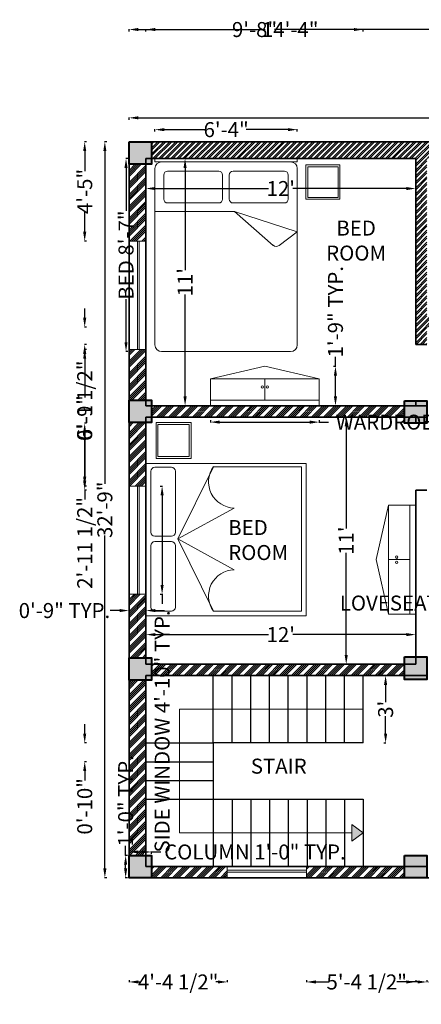
# Model space of a CAD drawing. Units: inches. Extents: x -52 to 493, y -432 to 100.
# Tile 1 of 5: x -52 to 163, y -432 to 94. Entities that reach past the tile are written whole.
import ezdxf

# ---------------------------------------------------------------- set-up
doc = ezdxf.new("R2010")
doc.units = ezdxf.units.IN
doc.header["$MEASUREMENT"] = 0
for name, color, linetype, lineweight in [('A-ANNO-DIMS', 2, 'Continuous', 18), ('A-ANNO-SYMB', 7, 'Continuous', 18), ('A-AREA-IDEN', 7, 'Continuous', 25), ('A-COLS', 7, 'Continuous', 40), ('A-FLOR-STRS', 7, 'Continuous', 25), ('A-FURN', 8, 'Continuous', 18), ('A-GLAZ', 4, 'Continuous', 18), ('A-WALL', 7, 'Continuous', 35), ('A-WALL-PATT', 8, 'Continuous', 13)]:
    doc.layers.add(name, color=color, linetype=linetype, lineweight=lineweight)
doc.styles.get("Standard").update_dxf_attribs({"font": 'arial.ttf'})
doc.dimstyles.get("Standard").update_dxf_attribs({"dimtxt": 8, "dimasz": 5, "dimexe": 0.18, "dimexo": 0.0625, "dimgap": 0.09, "dimtad": 0, "dimdec": 0, "dimzin": 0, "dimdsep": 46, "dimlunit": 3, "dimtxsty": 'Standard', "dimcen": 0.09, "dimadec": 0, "dimazin": 0, "dimtfac": 1, "dimtdec": 0, "dimtofl": 0, "dimtmove": 0, "dimatfit": 3, "dimfxl": 1, "dimfxlon": 1, "dimtolj": 1, "dimtzin": 0, "dimarcsym": 0})

# ---------------------------------------------------------------- blocks, each defined once
blk = doc.blocks.new('A$C400A1C0B')
for p, q in [((1.5, 2.035), (0, 2.035)), ((0, 2.035), (0, 2)), ((1.5, 2), (0, 2)), ((1.5, 2), (1.5, 2.035)), ((0, 1.93), (0, 0.07)), ((0.673, 1.902), (0.132, 1.902)), ((1.364, 1.902), (0.823, 1.902)), ((1.5, 0.07), (1.5, 1.93)), ((0.092, 1.862), (0.092, 1.607)), ((0.713, 1.607), (0.713, 1.862)), ((0.783, 1.862), (0.783, 1.607)), ((1.404, 1.607), (1.404, 1.862)), ((0.132, 1.567), (0.673, 1.567)), ((0.823, 1.567), (1.364, 1.567)), ((0.839, 1.476), (0, 1.476)), ((1.5, 1.261), (0.839, 1.476)), ((0.839, 1.476), (1.245, 1.12)), ((1.308, 1.117), (1.5, 1.261)), ((0.07, 0), (1.43, 0))]:
    blk.add_line(p, q)
for centre, radius, start, end in [((0.07, 1.93), 0.07, 90, 180), ((1.43, 1.93), 0.07, 0, 90), ((0.132, 1.862), 0.04, 90, 180), ((0.673, 1.862), 0.04, 0, 90), ((0.823, 1.862), 0.04, 90, 180), ((1.364, 1.862), 0.04, 0, 90), ((0.132, 1.607), 0.04, 180, 270), ((0.673, 1.607), 0.04, 270, 0), ((0.823, 1.607), 0.04, 180, 270), ((1.364, 1.607), 0.04, 270, 0), ((1.278, 1.158), 0.05, 228.6958, 306.7579), ((0.07, 0.07), 0.07, 180, 270), ((1.43, 0.07), 0.07, 270, 0)]:
    blk.add_arc(centre, radius, start, end)
blk = doc.blocks.new('A$C46517758')
for p, q in [((0, 0), (0, 2)), ((0, 2), (1.9, 2)), ((1.9, 2), (1.9, 0)), ((0.057, 1.888), (0.057, 1.682)), ((0.875, 1.938), (0.107, 1.938)), ((0.925, 1.682), (0.925, 1.888)), ((0.992, 1.682), (0.992, 1.888)), ((1.803, 1.938), (1.042, 1.938)), ((1.853, 1.682), (1.853, 1.888)), ((0.959, 1.602), (0.057, 1.156)), ((0.107, 1.632), (0.875, 1.632)), ((0.573, 0.898), (0.959, 1.602)), ((1.859, 1.156), (0.959, 1.602)), ((1.345, 0.898), (0.959, 1.602)), ((1.042, 1.632), (1.803, 1.632)), ((0.057, 1.156), (0.057, 0.057)), ((1.859, 0.057), (1.859, 1.156)), ((0.057, 0.057), (1.859, 0.057)), ((1.9, 0), (0, 0))]:
    blk.add_line(p, q)
for centre, radius, start, end in [((0.107, 1.888), 0.05, 90, 180), ((0.875, 1.888), 0.05, 0, 90), ((1.042, 1.888), 0.05, 90, 180), ((1.803, 1.888), 0.05, 0, 90), ((0.107, 1.682), 0.05, 180, 270), ((0.875, 1.682), 0.05, 270, 0), ((1.042, 1.682), 0.05, 180, 270), ((1.803, 1.682), 0.05, 270, 0), ((0.247, 0.892), 0.326, 1.0853, 125.715), ((1.671, 0.892), 0.326, 54.285, 178.9147)]:
    blk.add_arc(centre, radius, start, end)
blk = doc.blocks.new('*D11')
at = {"layer": 'A-ANNO-DIMS', "color": 0, "lineweight": -2, "transparency": 16777216}
for p, q in [((15.65, 2.39), (15.65, 3.57)), ((20.65, 3.39), (81.15, 3.39)), ((154.65, 3.39), (94.15, 3.39)), ((159.65, 2.39), (159.65, 3.57))]:
    blk.add_line(p, q, dxfattribs=at)
at = {"layer": 'A-ANNO-DIMS', "color": 0, "transparency": 16777216}
for points in [[(20.65, 4.23), (20.65, 2.56), (15.65, 3.39)], [(154.65, 4.23), (154.65, 2.56), (159.65, 3.39)]]:
    blk.add_solid(points, dxfattribs=at)
at = {"layer": 'Defpoints', "color": 0, "transparency": 16777216}
for p in [(159.65, 3.39), (15.65, -12.93), (159.65, -12.93)]:
    blk.add_point(p, dxfattribs=at)
at = {"layer": 'A-ANNO-DIMS', "color": 0, "transparency": 16777216, "insert": (87.65, 3.39), "char_height": 8, "attachment_point": 5}
blk.add_mtext("\\A1;12'", dxfattribs=at)
blk = doc.blocks.new('*D12')
at = {"layer": 'A-ANNO-DIMS', "color": 0, "lineweight": -2, "transparency": 16777216}
for p, q in [((35.57, 19.38), (36.75, 19.38)), ((36.57, 14.38), (36.57, -40.11)), ((36.57, -107.62), (36.57, -53.12)), ((35.57, -112.62), (36.75, -112.62))]:
    blk.add_line(p, q, dxfattribs=at)
at = {"layer": 'A-ANNO-DIMS', "color": 0, "transparency": 16777216}
for points in [[(35.74, 14.38), (37.4, 14.38), (36.57, 19.38)], [(35.74, -107.62), (37.4, -107.62), (36.57, -112.62)]]:
    blk.add_solid(points, dxfattribs=at)
at = {"layer": 'Defpoints', "color": 0, "transparency": 16777216}
for p in [(29.16, 19.38), (36.57, 19.38), (32.54, -112.62)]:
    blk.add_point(p, dxfattribs=at)
at = {"layer": 'A-ANNO-DIMS', "color": 0, "transparency": 16777216, "insert": (36.57, -46.62), "char_height": 8, "attachment_point": 5, "rotation": 90}
blk.add_mtext("\\A1;11'", dxfattribs=at)
blk = doc.blocks.new('*D17')
at = {"layer": 'A-ANNO-DIMS', "color": 0, "lineweight": -2, "transparency": 16777216}
for p, q in [((123.57, -118.62), (122.39, -118.62)), ((122.57, -123.62), (122.57, -178.11)), ((122.57, -245.62), (122.57, -191.12)), ((123.57, -250.62), (122.39, -250.62))]:
    blk.add_line(p, q, dxfattribs=at)
at = {"layer": 'A-ANNO-DIMS', "color": 0, "transparency": 16777216}
for points in [[(121.74, -123.62), (123.4, -123.62), (122.57, -118.62)], [(121.74, -245.62), (123.4, -245.62), (122.57, -250.62)]]:
    blk.add_solid(points, dxfattribs=at)
at = {"layer": 'Defpoints', "color": 0, "transparency": 16777216}
for p in [(122.57, -118.62), (129.39, -118.62), (129.39, -250.62)]:
    blk.add_point(p, dxfattribs=at)
at = {"layer": 'A-ANNO-DIMS', "color": 0, "transparency": 16777216, "insert": (122.57, -184.62), "char_height": 8, "attachment_point": 5, "rotation": 90}
blk.add_mtext("\\A1;11'", dxfattribs=at)
blk = doc.blocks.new('*D18')
at = {"layer": 'A-ANNO-DIMS', "color": 0, "lineweight": -2, "transparency": 16777216}
for p, q in [((15.65, -235.48), (15.65, -234.59)), ((20.65, -234.77), (81.15, -234.77)), ((154.65, -234.77), (94.15, -234.77)), ((159.65, -235.48), (159.65, -234.59))]:
    blk.add_line(p, q, dxfattribs=at)
at = {"layer": 'A-ANNO-DIMS', "color": 0, "transparency": 16777216}
for points in [[(20.65, -233.94), (20.65, -235.6), (15.65, -234.77)], [(154.65, -233.94), (154.65, -235.6), (159.65, -234.77)]]:
    blk.add_solid(points, dxfattribs=at)
at = {"layer": 'Defpoints', "color": 0, "transparency": 16777216}
for p in [(15.65, -234.77), (15.65, -235.55), (159.65, -235.55)]:
    blk.add_point(p, dxfattribs=at)
at = {"layer": 'A-ANNO-DIMS', "color": 0, "transparency": 16777216, "insert": (87.65, -234.77), "char_height": 8, "attachment_point": 5}
blk.add_mtext("\\A1;12'", dxfattribs=at)
blk = doc.blocks.new('*D21')
at = {"layer": 'A-ANNO-DIMS', "color": 0, "lineweight": -2, "transparency": 16777216}
for p, q in [((142.59, -256.62), (143.77, -256.62)), ((143.59, -261.62), (143.59, -270.85)), ((143.59, -287.62), (143.59, -278.38)), ((142.59, -292.62), (143.77, -292.62))]:
    blk.add_line(p, q, dxfattribs=at)
at = {"layer": 'A-ANNO-DIMS', "color": 0, "transparency": 16777216}
for points in [[(142.76, -261.62), (144.43, -261.62), (143.59, -256.62)], [(142.76, -287.62), (144.43, -287.62), (143.59, -292.62)]]:
    blk.add_solid(points, dxfattribs=at)
at = {"layer": 'Defpoints', "color": 0, "transparency": 16777216}
for p in [(131.65, -256.62), (143.59, -256.62), (131.65, -292.62)]:
    blk.add_point(p, dxfattribs=at)
at = {"layer": 'A-ANNO-DIMS', "color": 0, "transparency": 16777216, "insert": (143.59, -274.62), "char_height": 8, "attachment_point": 5, "rotation": 90}
blk.add_mtext("\\A1;3'", dxfattribs=at)
blk = doc.blocks.new('*D22')
at = {"layer": 'A-ANNO-DIMS', "color": 0, "lineweight": -2, "transparency": 16777216}
for p, q in [((6.65, 40.15), (6.65, 41.33)), ((11.65, 41.15), (179.77, 41.15)), ((361.65, 41.15), (193.52, 41.15)), ((366.65, 40.15), (366.65, 41.33))]:
    blk.add_line(p, q, dxfattribs=at)
at = {"layer": 'A-ANNO-DIMS', "color": 0, "transparency": 16777216}
for points in [[(11.65, 41.98), (11.65, 40.31), (6.65, 41.15)], [(361.65, 41.98), (361.65, 40.31), (366.65, 41.15)]]:
    blk.add_solid(points, dxfattribs=at)
at = {"layer": 'Defpoints', "color": 0, "transparency": 16777216}
for p in [(366.65, 41.15), (6.65, 28.38), (366.65, 28.38)]:
    blk.add_point(p, dxfattribs=at)
at = {"layer": 'A-ANNO-DIMS', "color": 0, "transparency": 16777216, "insert": (186.65, 41.15), "char_height": 8, "attachment_point": 5}
blk.add_mtext("\\A1;30'", dxfattribs=at)
blk = doc.blocks.new('*D23')
at = {"layer": 'A-ANNO-DIMS', "color": 0, "lineweight": -2, "transparency": 16777216}
for p, q in [((-5.25, 28.38), (-6.43, 28.38)), ((-6.25, 23.38), (-6.25, -154.29)), ((-6.25, -359.62), (-6.25, -181.94)), ((-5.25, -364.62), (-6.43, -364.62))]:
    blk.add_line(p, q, dxfattribs=at)
at = {"layer": 'A-ANNO-DIMS', "color": 0, "transparency": 16777216}
for points in [[(-7.08, 23.38), (-5.42, 23.38), (-6.25, 28.38)], [(-7.08, -359.62), (-5.42, -359.62), (-6.25, -364.62)]]:
    blk.add_solid(points, dxfattribs=at)
at = {"layer": 'Defpoints', "color": 0, "transparency": 16777216}
for p in [(6.65, 28.38), (-6.25, -364.62), (6.65, -364.62)]:
    blk.add_point(p, dxfattribs=at)
at = {"layer": 'A-ANNO-DIMS', "color": 0, "transparency": 16777216, "insert": (-6.25, -168.12), "char_height": 8, "attachment_point": 5, "rotation": 90}
blk.add_mtext('\\A1;32\'-9"', dxfattribs=at)
blk = doc.blocks.new('COL-12X12')
h = blk.add_hatch(color=256)
h.dxf.hatch_style = 1
h.paths.add_polyline_path([(12, 12), (0, 12), (0, 0), (12, 0)])
blk.add_lwpolyline([(0, 12), (12, 12), (12, 0), (0, 0)], close=True)
blk = doc.blocks.new('WIN-SIDE-58')
for p, q in [((0, 57.79), (9, 57.79)), ((3.5, 0), (3.5, 57.79)), ((4.5, 0), (4.5, 57.79)), ((0, 0), (9, 0))]:
    blk.add_line(p, q)
blk = doc.blocks.new('WIN-FRONT-42')
for p, q in [((0, 6), (0, 0)), ((42.31, 6), (42.31, 0)), ((42.31, 4), (0, 4)), ((42.31, 3), (0, 3))]:
    blk.add_line(p, q)
blk = doc.blocks.new('WARDROBE-DOUBLE')
for p, q in [((0, 14.42), (29.03, 21.14)), ((29.03, 21.14), (58.05, 14.42)), ((0, 3.04), (0, 14.42)), ((0, 14.42), (58.05, 14.42)), ((29.03, 14.42), (29.03, 3.04)), ((58.05, 14.42), (58.05, 3.04)), ((0, 0), (0, 3.04)), ((0, 3.04), (58.05, 3.04)), ((58.05, 3.04), (58.05, 0))]:
    blk.add_line(p, q)
for centre in [(27.68, 10.11), (30.45, 10.11)]:
    blk.add_circle(centre, 0.653)
blk = doc.blocks.new('*D32')
at = {"layer": 'A-ANNO-DIMS', "color": 0, "lineweight": -2, "transparency": 16777216}
for p, q in [((6.65, -351.82), (6.65, -350.64)), ((11.65, -350.82), (13.65, -350.82)), ((18.65, -351.82), (18.65, -350.64)), ((18.65, -350.82), (23.65, -350.82))]:
    blk.add_line(p, q, dxfattribs=at)
at = {"layer": 'A-ANNO-DIMS', "color": 0, "transparency": 16777216}
for points in [[(11.65, -349.98), (11.65, -351.65), (6.65, -350.82)], [(13.65, -349.98), (13.65, -351.65), (18.65, -350.82)]]:
    blk.add_solid(points, dxfattribs=at)
at = {"layer": 'Defpoints', "color": 0, "transparency": 16777216}
for p in [(18.65, -350.82), (6.65, -352.62), (18.65, -352.62)]:
    blk.add_point(p, dxfattribs=at)
at = {"layer": 'A-ANNO-DIMS', "color": 0, "transparency": 16777216, "insert": (73.84, -350.82), "char_height": 8, "attachment_point": 5}
blk.add_mtext('\\A1;COLUMN 1\'-0" TYP.', dxfattribs=at)
blk = doc.blocks.new('*D33')
at = {"layer": 'A-ANNO-DIMS', "color": 0, "lineweight": -2, "transparency": 16777216}
for p, q in [((4.85, -352.62), (4.85, -347.62)), ((5.85, -352.62), (4.67, -352.62)), ((4.85, -359.62), (4.85, -357.62)), ((5.85, -364.62), (4.67, -364.62))]:
    blk.add_line(p, q, dxfattribs=at)
at = {"layer": 'A-ANNO-DIMS', "color": 0, "transparency": 16777216}
for points in [[(4.01, -357.62), (5.68, -357.62), (4.85, -352.62)], [(4.01, -359.62), (5.68, -359.62), (4.85, -364.62)]]:
    blk.add_solid(points, dxfattribs=at)
at = {"layer": 'Defpoints', "color": 0, "transparency": 16777216}
for p in [(4.85, -352.62), (6.65, -352.62), (6.65, -364.62)]:
    blk.add_point(p, dxfattribs=at)
at = {"layer": 'A-ANNO-DIMS', "color": 0, "transparency": 16777216, "insert": (4.85, -323.52), "char_height": 8, "attachment_point": 5, "rotation": 90}
blk.add_mtext('\\A1;1\'-0" TYP.', dxfattribs=at)
blk = doc.blocks.new('*D34')
at = {"layer": 'A-ANNO-DIMS', "color": 0, "lineweight": -2, "transparency": 16777216}
for p, q in [((23.32, -155.46), (24.5, -155.46)), ((24.32, -160.46), (24.32, -208.25)), ((23.32, -213.25), (24.5, -213.25)), ((24.32, -213.25), (24.32, -218.25))]:
    blk.add_line(p, q, dxfattribs=at)
at = {"layer": 'A-ANNO-DIMS', "color": 0, "transparency": 16777216}
for points in [[(23.48, -160.46), (25.15, -160.46), (24.32, -155.46)], [(23.48, -208.25), (25.15, -208.25), (24.32, -213.25)]]:
    blk.add_solid(points, dxfattribs=at)
at = {"layer": 'Defpoints', "color": 0, "transparency": 16777216}
for p in [(15.65, -155.46), (15.65, -213.25), (24.32, -213.25)]:
    blk.add_point(p, dxfattribs=at)
at = {"layer": 'A-ANNO-DIMS', "color": 0, "transparency": 16777216, "insert": (24.32, -286.48), "char_height": 8, "attachment_point": 5, "rotation": 90}
blk.add_mtext('\\A1;SIDE WINDOW 4\'-10" TYP.', dxfattribs=at)
blk = doc.blocks.new('*D35')
at = {"layer": 'A-ANNO-DIMS', "color": 0, "lineweight": -2, "transparency": 16777216}
for p, q in [((1.65, -221.92), (-3.35, -221.92)), ((6.65, -220.92), (6.65, -222.1)), ((15.65, -220.92), (15.65, -222.1)), ((20.65, -221.92), (25.65, -221.92))]:
    blk.add_line(p, q, dxfattribs=at)
at = {"layer": 'A-ANNO-DIMS', "color": 0, "transparency": 16777216}
for points in [[(1.65, -221.09), (1.65, -222.76), (6.65, -221.92)], [(20.65, -221.09), (20.65, -222.76), (15.65, -221.92)]]:
    blk.add_solid(points, dxfattribs=at)
at = {"layer": 'Defpoints', "color": 0, "transparency": 16777216}
for p in [(6.65, -213.25), (15.65, -213.25), (6.65, -221.92)]:
    blk.add_point(p, dxfattribs=at)
at = {"layer": 'A-ANNO-DIMS', "color": 0, "transparency": 16777216, "insert": (-27.82, -221.92), "char_height": 8, "attachment_point": 5}
blk.add_mtext('\\A1;0\'-9" TYP.', dxfattribs=at)
blk = doc.blocks.new('*D38')
at = {"layer": 'A-ANNO-DIMS', "color": 0, "lineweight": -2, "transparency": 16777216}
for p, q in [((50.07, -120.32), (50.07, -121.5)), ((108.12, -120.32), (108.12, -121.5)), ((55.07, -121.32), (103.12, -121.32)), ((108.12, -121.32), (113.12, -121.32))]:
    blk.add_line(p, q, dxfattribs=at)
at = {"layer": 'A-ANNO-DIMS', "color": 0, "transparency": 16777216}
for points in [[(55.07, -120.49), (55.07, -122.16), (50.07, -121.32)], [(103.12, -120.49), (103.12, -122.16), (108.12, -121.32)]]:
    blk.add_solid(points, dxfattribs=at)
at = {"layer": 'Defpoints', "color": 0, "transparency": 16777216}
for p in [(50.07, -112.62), (108.12, -112.62), (108.12, -121.32)]:
    blk.add_point(p, dxfattribs=at)
at = {"layer": 'A-ANNO-DIMS', "color": 0, "transparency": 16777216, "insert": (175.33, -121.32), "char_height": 8, "attachment_point": 5}
blk.add_mtext('\\A1;WARDROBE 4\'-10" TYP.', dxfattribs=at)
blk = doc.blocks.new('*D39')
at = {"layer": 'A-ANNO-DIMS', "color": 0, "lineweight": -2, "transparency": 16777216}
for p, q in [((116.83, -91.48), (116.83, -86.48)), ((115.83, -91.48), (117.01, -91.48)), ((116.83, -107.62), (116.83, -96.48)), ((115.83, -112.62), (117.01, -112.62))]:
    blk.add_line(p, q, dxfattribs=at)
at = {"layer": 'A-ANNO-DIMS', "color": 0, "transparency": 16777216}
for points in [[(116, -96.48), (117.66, -96.48), (116.83, -91.48)], [(116, -107.62), (117.66, -107.62), (116.83, -112.62)]]:
    blk.add_solid(points, dxfattribs=at)
at = {"layer": 'Defpoints', "color": 0, "transparency": 16777216}
for p in [(108.12, -91.48), (116.83, -91.48), (108.12, -112.62)]:
    blk.add_point(p, dxfattribs=at)
at = {"layer": 'A-ANNO-DIMS', "color": 0, "transparency": 16777216, "insert": (116.83, -62.38), "char_height": 8, "attachment_point": 5, "rotation": 90}
blk.add_mtext('\\A1;1\'-9" TYP.', dxfattribs=at)
blk = doc.blocks.new('*D40')
at = {"layer": 'A-ANNO-DIMS', "color": 0, "lineweight": -2, "transparency": 16777216}
for p, q in [((6.05, 19.38), (4.87, 19.38)), ((5.05, 14.38), (5.05, -8.55)), ((5.05, -78.66), (5.05, -55.73)), ((6.05, -83.66), (4.87, -83.66))]:
    blk.add_line(p, q, dxfattribs=at)
at = {"layer": 'A-ANNO-DIMS', "color": 0, "transparency": 16777216}
for points in [[(4.22, 14.38), (5.89, 14.38), (5.05, 19.38)], [(4.22, -78.66), (5.89, -78.66), (5.05, -83.66)]]:
    blk.add_solid(points, dxfattribs=at)
at = {"layer": 'Defpoints', "color": 0, "transparency": 16777216}
for p in [(5.05, 19.38), (20.51, 19.38), (20.51, -83.66)]:
    blk.add_point(p, dxfattribs=at)
at = {"layer": 'A-ANNO-DIMS', "color": 0, "transparency": 16777216, "insert": (5.05, -32.14), "char_height": 8, "attachment_point": 5, "rotation": 90}
blk.add_mtext('\\A1;BED 8\'-7"', dxfattribs=at)
blk = doc.blocks.new('*D41')
at = {"layer": 'A-ANNO-DIMS', "color": 0, "lineweight": -2, "transparency": 16777216}
for p, q in [((20.51, 33.84), (20.51, 35.02)), ((25.51, 34.84), (47.74, 34.84)), ((91.46, 34.84), (69.23, 34.84)), ((96.46, 33.84), (96.46, 35.02))]:
    blk.add_line(p, q, dxfattribs=at)
at = {"layer": 'A-ANNO-DIMS', "color": 0, "transparency": 16777216}
for points in [[(25.51, 35.67), (25.51, 34.01), (20.51, 34.84)], [(91.46, 35.67), (91.46, 34.01), (96.46, 34.84)]]:
    blk.add_solid(points, dxfattribs=at)
at = {"layer": 'Defpoints', "color": 0, "transparency": 16777216}
for p in [(96.46, 34.84), (20.51, 19.38), (96.46, 19.38)]:
    blk.add_point(p, dxfattribs=at)
at = {"layer": 'A-ANNO-DIMS', "color": 0, "transparency": 16777216, "insert": (58.49, 34.84), "char_height": 8, "attachment_point": 5}
blk.add_mtext('\\A1;6\'-4"', dxfattribs=at)
blk = doc.blocks.new('*D50')
at = {"layer": 'A-ANNO-DIMS', "color": 0, "lineweight": -2, "transparency": 16777216}
for p, q in [((205.43, -217.92), (200.43, -217.92)), ((205.43, -218.92), (205.43, -217.74)), ((237.52, -217.92), (210.43, -217.92)), ((242.52, -218.92), (242.52, -217.74))]:
    blk.add_line(p, q, dxfattribs=at)
at = {"layer": 'A-ANNO-DIMS', "color": 0, "transparency": 16777216}
for points in [[(210.43, -217.09), (210.43, -218.75), (205.43, -217.92)], [(237.52, -217.09), (237.52, -218.75), (242.52, -217.92)]]:
    blk.add_solid(points, dxfattribs=at)
at = {"layer": 'Defpoints', "color": 0, "transparency": 16777216}
for p in [(205.43, -217.92), (205.43, -223.48), (242.52, -223.48)]:
    blk.add_point(p, dxfattribs=at)
at = {"layer": 'A-ANNO-DIMS', "color": 0, "transparency": 16777216, "insert": (158.83, -217.92), "char_height": 8, "attachment_point": 5}
blk.add_mtext('\\A1;LOVESEAT 3\'-1"', dxfattribs=at)
blk = doc.blocks.new('*D56')
at = {"layer": 'A-ANNO-DIMS', "color": 0, "lineweight": -2, "transparency": 16777216}
for p, q in [((6.65, 87.29), (6.65, 88.47)), ((11.65, 88.29), (79.23, 88.29)), ((173.72, 88.29), (106.14, 88.29)), ((178.72, 87.29), (178.72, 88.47))]:
    blk.add_line(p, q, dxfattribs=at)
at = {"layer": 'A-ANNO-DIMS', "color": 0, "transparency": 16777216}
for points in [[(11.65, 89.13), (11.65, 87.46), (6.65, 88.29)], [(173.72, 89.13), (173.72, 87.46), (178.72, 88.29)]]:
    blk.add_solid(points, dxfattribs=at)
at = {"layer": 'Defpoints', "color": 0, "transparency": 16777216}
for p in [(178.72, 88.29), (6.65, 28.38), (178.72, 28.38)]:
    blk.add_point(p, dxfattribs=at)
at = {"layer": 'A-ANNO-DIMS', "color": 0, "transparency": 16777216, "insert": (92.68, 88.29), "char_height": 8, "attachment_point": 5}
blk.add_mtext('\\A1;14\'-4"', dxfattribs=at)
blk = doc.blocks.new('*D60')
at = {"layer": 'A-ANNO-DIMS', "color": 0, "lineweight": -2, "transparency": 16777216}
for p, q in [((-16, 28.38), (-17.18, 28.38)), ((-17, 23.38), (-17, 12.72)), ((-17, -19.71), (-17, -9.05)), ((-16, -24.71), (-17.18, -24.71))]:
    blk.add_line(p, q, dxfattribs=at)
at = {"layer": 'A-ANNO-DIMS', "color": 0, "transparency": 16777216}
for points in [[(-17.84, 23.38), (-16.17, 23.38), (-17, 28.38)], [(-17.84, -19.71), (-16.17, -19.71), (-17, -24.71)]]:
    blk.add_solid(points, dxfattribs=at)
at = {"layer": 'Defpoints', "color": 0, "transparency": 16777216}
for p in [(6.65, 28.38), (-17, -24.71), (6.65, -24.71)]:
    blk.add_point(p, dxfattribs=at)
at = {"layer": 'A-ANNO-DIMS', "color": 0, "transparency": 16777216, "insert": (-17, 1.84), "char_height": 8, "attachment_point": 5, "rotation": 90}
blk.add_mtext('\\A1;4\'-5"', dxfattribs=at)
blk = doc.blocks.new('*D61')
at = {"layer": 'A-ANNO-DIMS', "color": 0, "lineweight": -2, "transparency": 16777216}
for p, q in [((-16, -82.5), (-17.18, -82.5)), ((-17, -87.5), (-17, -108.24)), ((-17, -150.46), (-17, -129.73)), ((-16, -155.46), (-17.18, -155.46))]:
    blk.add_line(p, q, dxfattribs=at)
at = {"layer": 'A-ANNO-DIMS', "color": 0, "transparency": 16777216}
for points in [[(-17.84, -87.5), (-16.17, -87.5), (-17, -82.5)], [(-17.84, -150.46), (-16.17, -150.46), (-17, -155.46)]]:
    blk.add_solid(points, dxfattribs=at)
at = {"layer": 'Defpoints', "color": 0, "transparency": 16777216}
for p in [(6.65, -82.5), (-17, -155.46), (6.65, -155.46)]:
    blk.add_point(p, dxfattribs=at)
at = {"layer": 'A-ANNO-DIMS', "color": 0, "transparency": 16777216, "insert": (-17, -118.98), "char_height": 8, "attachment_point": 5, "rotation": 90}
blk.add_mtext('\\A1;6\'-1"', dxfattribs=at)
blk = doc.blocks.new('*D63')
at = {"layer": 'A-ANNO-DIMS', "color": 0, "lineweight": -2, "transparency": 16777216}
for p, q in [((6.65, -419.22), (6.65, -420.4)), ((11.65, -420.22), (12.66, -420.22)), ((54.09, -420.22), (53.07, -420.22)), ((59.09, -419.22), (59.09, -420.4))]:
    blk.add_line(p, q, dxfattribs=at)
at = {"layer": 'A-ANNO-DIMS', "color": 0, "transparency": 16777216}
for points in [[(11.65, -419.39), (11.65, -421.06), (6.65, -420.22)], [(54.09, -419.39), (54.09, -421.06), (59.09, -420.22)]]:
    blk.add_solid(points, dxfattribs=at)
at = {"layer": 'Defpoints', "color": 0, "transparency": 16777216}
for p in [(6.65, -364.62), (59.09, -364.62), (59.09, -420.22)]:
    blk.add_point(p, dxfattribs=at)
at = {"layer": 'A-ANNO-DIMS', "color": 0, "transparency": 16777216, "insert": (32.87, -420.22), "char_height": 8, "attachment_point": 5}
blk.add_mtext('\\A1;4\'-4 1/2"', dxfattribs=at)
blk = doc.blocks.new('*D64')
at = {"layer": 'A-ANNO-DIMS', "color": 0, "lineweight": -2, "transparency": 16777216}
for p, q in [((101.4, -419.22), (101.4, -420.4)), ((106.4, -420.22), (113.48, -420.22)), ((160.65, -420.22), (153.57, -420.22)), ((165.65, -419.22), (165.65, -420.4))]:
    blk.add_line(p, q, dxfattribs=at)
at = {"layer": 'A-ANNO-DIMS', "color": 0, "transparency": 16777216}
for points in [[(106.4, -419.39), (106.4, -421.06), (101.4, -420.22)], [(160.65, -419.39), (160.65, -421.06), (165.65, -420.22)]]:
    blk.add_solid(points, dxfattribs=at)
at = {"layer": 'Defpoints', "color": 0, "transparency": 16777216}
for p in [(101.4, -364.62), (165.65, -364.62), (165.65, -420.22)]:
    blk.add_point(p, dxfattribs=at)
at = {"layer": 'A-ANNO-DIMS', "color": 0, "transparency": 16777216, "insert": (133.52, -420.22), "char_height": 8, "attachment_point": 5}
blk.add_mtext('\\A1;5\'-4 1/2"', dxfattribs=at)
blk = doc.blocks.new('*D68')
at = {"layer": 'A-ANNO-DIMS', "color": 0, "lineweight": -2, "transparency": 16777216}
for p, q in [((-17, -287.62), (-17, -282.62)), ((-16, -292.62), (-17.18, -292.62)), ((-16, -302.62), (-17.18, -302.62)), ((-17, -307.62), (-17, -312.62))]:
    blk.add_line(p, q, dxfattribs=at)
at = {"layer": 'A-ANNO-DIMS', "color": 0, "transparency": 16777216}
for points in [[(-17.84, -287.62), (-16.17, -287.62), (-17, -292.62)], [(-17.84, -307.62), (-16.17, -307.62), (-17, -302.62)]]:
    blk.add_solid(points, dxfattribs=at)
at = {"layer": 'Defpoints', "color": 0, "transparency": 16777216}
for p in [(15.65, -292.62), (-17, -302.62), (15.65, -302.62)]:
    blk.add_point(p, dxfattribs=at)
at = {"layer": 'A-ANNO-DIMS', "color": 0, "transparency": 16777216, "insert": (-17, -326.45), "char_height": 8, "attachment_point": 5, "rotation": 90}
blk.add_mtext('\\A1;0\'-10"', dxfattribs=at)
blk = doc.blocks.new('*D69')
at = {"layer": 'A-ANNO-DIMS', "color": 0, "lineweight": -2, "transparency": 16777216}
for p, q in [((15.65, 87.29), (15.65, 88.47)), ((20.65, 88.29), (62.92, 88.29)), ((126.65, 88.29), (84.37, 88.29)), ((131.65, 87.29), (131.65, 88.47))]:
    blk.add_line(p, q, dxfattribs=at)
at = {"layer": 'A-ANNO-DIMS', "color": 0, "transparency": 16777216}
for points in [[(20.65, 89.13), (20.65, 87.46), (15.65, 88.29)], [(126.65, 89.13), (126.65, 87.46), (131.65, 88.29)]]:
    blk.add_solid(points, dxfattribs=at)
at = {"layer": 'Defpoints', "color": 0, "transparency": 16777216}
for p in [(131.65, 88.29), (15.65, -256.62), (131.65, -256.62)]:
    blk.add_point(p, dxfattribs=at)
at = {"layer": 'A-ANNO-DIMS', "color": 0, "transparency": 16777216, "insert": (73.65, 88.29), "char_height": 8, "attachment_point": 5}
blk.add_mtext('\\A1;9\'-8"', dxfattribs=at)
blk = doc.blocks.new('*D71')
at = {"layer": 'A-ANNO-DIMS', "color": 0, "lineweight": -2, "transparency": 16777216}
for p, q in [((-17, -65.62), (-17, -60.62)), ((-16, -70.62), (-17.18, -70.62)), ((-16, -79.87), (-17.18, -79.87)), ((-17, -84.87), (-17, -89.87))]:
    blk.add_line(p, q, dxfattribs=at)
at = {"layer": 'A-ANNO-DIMS', "color": 0, "transparency": 16777216}
for points in [[(-17.84, -65.62), (-16.17, -65.62), (-17, -70.62)], [(-17.84, -84.87), (-16.17, -84.87), (-17, -79.87)]]:
    blk.add_solid(points, dxfattribs=at)
at = {"layer": 'Defpoints', "color": 0, "transparency": 16777216}
for p in [(165.65, -70.62), (-17, -79.87), (165.65, -79.87)]:
    blk.add_point(p, dxfattribs=at)
at = {"layer": 'A-ANNO-DIMS', "color": 0, "transparency": 16777216, "insert": (-17, -109.92), "char_height": 8, "attachment_point": 5, "rotation": 90}
blk.add_mtext('\\A1;0\'-9 1/2"', dxfattribs=at)
blk = doc.blocks.new('*D72')
at = {"layer": 'A-ANNO-DIMS', "color": 0, "lineweight": -2, "transparency": 16777216}
for p, q in [((-16, -121.95), (-17.18, -121.95)), ((-17, -126.95), (-17, -152.57)), ((-16, -157.57), (-17.18, -157.57)), ((-17, -157.57), (-17, -162.57))]:
    blk.add_line(p, q, dxfattribs=at)
at = {"layer": 'A-ANNO-DIMS', "color": 0, "transparency": 16777216}
for points in [[(-17.84, -126.95), (-16.17, -126.95), (-17, -121.95)], [(-17.84, -152.57), (-16.17, -152.57), (-17, -157.57)]]:
    blk.add_solid(points, dxfattribs=at)
at = {"layer": 'Defpoints', "color": 0, "transparency": 16777216}
for p in [(159.65, -121.95), (-17, -157.57), (159.65, -157.57)]:
    blk.add_point(p, dxfattribs=at)
at = {"layer": 'A-ANNO-DIMS', "color": 0, "transparency": 16777216, "insert": (-17, -185.79), "char_height": 8, "attachment_point": 5, "rotation": 90}
blk.add_mtext('\\A1;2\'-11 1/2"', dxfattribs=at)
blk = doc.blocks.new('*D81')
at = {"layer": 'A-ANNO-DIMS', "color": 0, "lineweight": -2, "transparency": 16777216}
for p, q in [((154.65, -420.22), (149.65, -420.22)), ((159.65, -419.22), (159.65, -420.4)), ((165.65, -419.22), (165.65, -420.4)), ((170.65, -420.22), (175.65, -420.22))]:
    blk.add_line(p, q, dxfattribs=at)
at = {"layer": 'A-ANNO-DIMS', "color": 0, "transparency": 16777216}
for points in [[(154.65, -419.39), (154.65, -421.06), (159.65, -420.22)], [(170.65, -419.39), (170.65, -421.06), (165.65, -420.22)]]:
    blk.add_solid(points, dxfattribs=at)
at = {"layer": 'Defpoints', "color": 0, "transparency": 16777216}
for p in [(159.65, -79.87), (165.65, -79.87), (165.65, -420.22)]:
    blk.add_point(p, dxfattribs=at)
at = {"layer": 'A-ANNO-DIMS', "color": 0, "transparency": 16777216, "insert": (186.37, -420.22), "char_height": 8, "attachment_point": 5}
blk.add_mtext('\\A1;0\'-6"', dxfattribs=at)

msp = doc.modelspace()

# ---------------------------------------------------------------- hatches: boundary and pattern name
at = {"layer": 'A-ANNO-SYMB'}
h = msp.add_hatch(color=256, dxfattribs=at)
h.dxf.hatch_style = 1
h.paths.add_polyline_path([(131.65, -340.62), (125.61, -336.23), (125.61, -340.62), (125.61, -345)])
at = {"layer": 'A-WALL-PATT'}
h = msp.add_hatch(dxfattribs=at)
h.set_pattern_fill('ANSI32', color=256, scale=6)
h.paths.add_polyline_path([(178.72, 28.38), (18.65, 28.38), (18.65, 19.38), (159.65, 19.38), (159.65, -79.87), (165.65, -79.87), (165.65, -70.62), (213.65, -70.62), (213.65, -79.87), (219.65, -79.87), (219.65, 19.38), (260.34, 19.38), (260.34, 28.38), (205.54, 28.38), (205.54, 19.38), (213.65, 19.38), (213.65, -64.62), (165.65, -64.62), (165.65, 19.38), (178.72, 19.38)])
h.paths.add_polyline_path([(354.65, 28.38), (309.11, 28.38), (309.11, 19.38), (354.65, 19.38)])
h = msp.add_hatch(dxfattribs=at)
h.set_pattern_fill('ANSI34', color=256, scale=6)
h.paths.add_polyline_path([(366.65, 16.38), (357.65, 16.38), (357.65, -110.87), (366.65, -110.87)])
h.paths.add_polyline_path([(15.65, 16.38), (6.65, 16.38), (6.65, -24.71), (15.65, -24.71)])
h.paths.add_polyline_path([(15.65, -82.5), (6.65, -82.5), (6.65, -109.57), (15.65, -109.57)])
h.paths.add_polyline_path([(366.65, -122.87), (357.65, -122.87), (357.65, -155.46), (366.65, -155.46)])
h.paths.add_polyline_path([(354.65, -112.62), (225.65, -112.62), (225.65, -118.62), (354.65, -118.62)])
h.paths.add_polyline_path([(153.65, -112.62), (18.65, -112.62), (18.65, -118.62), (153.65, -118.62)])
h = msp.add_hatch(dxfattribs=at)
h.set_pattern_fill('ANSI34', color=256, scale=6)
h.paths.add_polyline_path([(366.65, -213.25), (357.65, -213.25), (357.65, -247.89), (366.65, -247.89)])
h.paths.add_polyline_path([(354.65, -250.62), (267.65, -250.62), (267.65, -256.62), (354.65, -256.62)])
h.paths.add_polyline_path([(366.65, -259.89), (357.65, -259.89), (357.65, -352.62), (366.65, -352.62)])
h.paths.add_polyline_path([(354.65, -358.62), (331.2, -358.62), (331.2, -364.62), (354.65, -364.62)])
h.paths.add_polyline_path([(288.89, -358.62), (267.65, -358.62), (267.65, -364.62), (288.89, -364.62)])
h.paths.add_polyline_path([(153.65, -358.62), (101.4, -358.62), (101.4, -364.62), (153.65, -364.62)])
h.paths.add_polyline_path([(59.09, -358.62), (18.65, -358.62), (18.65, -364.62), (59.09, -364.62)])
h.paths.add_polyline_path([(15.65, -259.14), (6.65, -259.14), (6.65, -352.62), (15.65, -352.62)])
h.paths.add_polyline_path([(153.65, -250.62), (18.65, -250.62), (18.65, -256.62), (153.65, -256.62)])
h.paths.add_polyline_path([(15.65, -213.25), (6.65, -213.25), (6.65, -247.14), (15.65, -247.14)])
h.paths.add_polyline_path([(15.65, -121.57), (6.65, -121.57), (6.65, -155.46), (15.65, -155.46), (15.65, -143.44)])

# ---------------------------------------------------------------- linework, layer by layer
at = {"layer": 'A-ANNO-SYMB'}
for p, q in [((51.65, -274.62), (33.65, -274.62)), ((33.65, -274.62), (33.65, -340.62)), ((131.65, -274.62), (51.65, -274.62)), ((125.61, -340.62), (125.61, -336.23)), ((125.61, -336.23), (131.65, -340.62)), ((33.65, -340.62), (121.65, -340.62)), ((121.65, -340.62), (125.61, -340.62)), ((125.61, -340.62), (125.61, -345)), ((125.61, -345), (131.65, -340.62))]:
    msp.add_line(p, q, dxfattribs=at)
at = {"layer": 'A-FLOR-STRS'}
for p, q in [((51.65, -292.62), (51.65, -256.62)), ((61.65, -292.62), (61.65, -256.62)), ((71.65, -292.62), (71.65, -256.62)), ((81.65, -292.62), (81.65, -256.62)), ((91.65, -292.62), (91.65, -256.62)), ((101.65, -292.62), (101.65, -256.62)), ((111.65, -292.62), (111.65, -256.62)), ((121.65, -292.62), (121.65, -256.62)), ((131.65, -292.62), (131.65, -256.62)), ((15.65, -292.62), (51.65, -292.62)), ((15.65, -292.62), (51.65, -292.62)), ((131.65, -292.62), (51.65, -292.62)), ((51.65, -292.62), (51.65, -322.62)), ((15.65, -302.62), (51.65, -302.62)), ((15.65, -312.62), (51.65, -312.62)), ((15.65, -322.62), (51.65, -322.62)), ((51.65, -322.62), (51.65, -358.62)), ((51.65, -322.62), (131.65, -322.62)), ((61.65, -322.62), (61.65, -358.62)), ((71.65, -322.62), (71.65, -358.62)), ((81.65, -322.62), (81.65, -358.62)), ((91.65, -322.62), (91.65, -358.62)), ((101.65, -322.62), (101.65, -358.62)), ((111.65, -322.62), (111.65, -358.62)), ((121.65, -322.62), (121.65, -358.62)), ((131.65, -322.62), (131.65, -358.62))]:
    msp.add_line(p, q, dxfattribs=at)
at = {"layer": 'A-FURN'}
for points in [[(101, 16.01), (119.25, 16.01), (119.25, -2.35), (101, -2.35)], [(102, 15.01), (118.25, 15.01), (118.25, -1.35), (102, -1.35)], [(21.09, -121.58), (39.84, -121.58), (39.84, -140.72), (21.09, -140.72)], [(22.09, -122.58), (38.84, -122.58), (38.84, -139.72), (22.09, -139.72)]]:
    msp.add_lwpolyline(points, close=True, dxfattribs=at)
at = {"layer": 'A-WALL'}
for p, q in [((6.65, 28.38), (366.65, 28.38)), ((6.65, 28.38), (6.65, -364.62)), ((15.65, 19.38), (159.65, 19.38)), ((15.65, 19.38), (15.65, -112.62)), ((159.65, 19.38), (159.65, -79.87)), ((165.65, -79.87), (159.65, -79.87)), ((159.65, -109.95), (159.65, -112.62)), ((15.65, -112.62), (159.65, -112.62)), ((159.65, -112.62), (165.65, -112.62)), ((15.65, -118.62), (159.65, -118.62)), ((15.65, -118.62), (15.65, -250.62)), ((159.65, -118.62), (165.65, -118.62)), ((159.65, -118.62), (159.65, -121.95)), ((165.65, -157.57), (159.65, -157.57)), ((159.65, -157.57), (159.65, -250.62)), ((15.65, -250.62), (159.65, -250.62)), ((15.65, -256.62), (165.65, -256.62)), ((15.65, -256.62), (15.65, -358.62)), ((15.65, -358.62), (165.65, -358.62)), ((6.65, -364.62), (366.65, -364.62))]:
    msp.add_line(p, q, dxfattribs=at)

# ---------------------------------------------------------------- block references
at = {"layer": 'A-COLS'}
for p in [(6.65, 16.38), (6.65, -121.57), (153.65, -121.95), (153.65, -258.71), (6.65, -259.14), (6.65, -364.62), (153.65, -364.62)]:
    msp.add_blockref('COL-12X12', p, dxfattribs=at)
at = {"layer": 'A-FURN', "xscale": 50.63501003620931, "yscale": 50.63501003620931, "zscale": 50.63501003620931}
msp.add_blockref('A$C400A1C0B', (20.51, -83.66), dxfattribs=at)
at = {"layer": 'A-FURN'}
msp.add_blockref('WARDROBE-DOUBLE', (50.07, -112.62), dxfattribs=at)
at = {"layer": 'A-FURN', "xscale": 42.76422276661556, "yscale": 42.76422276661556, "zscale": 42.76422276661556, "rotation": 90}
msp.add_blockref('A$C46517758', (101.18, -224.69), dxfattribs=at)
at = {"layer": 'A-FURN', "extrusion": (0, 0, -1), "zscale": -1, "rotation": 269.9999999999999}
msp.add_blockref('WARDROBE-DOUBLE', (-159.65, -165.72), dxfattribs=at)
at = {"layer": 'A-GLAZ', "rotation": 180}
for p in [(15.65, -24.71), (15.65, -155.46)]:
    msp.add_blockref('WIN-SIDE-58', p, dxfattribs=at)
at = {"layer": 'A-GLAZ'}
msp.add_blockref('WIN-FRONT-42', (59.09, -364.62), dxfattribs=at)

# ---------------------------------------------------------------- texts
at = {"layer": 'A-AREA-IDEN', "char_height": 8, "attachment_point": 1}
for s, width, insert in [('\\pxqc;BED\\PROOM', 42.7825, (106.48, -13.73)), ('BED\\PROOM', 75.9525, (59.6, -173.61)), ('STAIR', 75.9525, (71.65, -301))]:
    msp.add_mtext_dynamic_manual_height_columns(s, width=width, gutter_width=1, heights=[0], dxfattribs=dict(at, insert=insert))

# ---------------------------------------------------------------- dimensions: what is measured, and where the dimension line sits
at = {"layer": 'A-ANNO-DIMS'}
for base, p1, p2, override, picture, middle in [((178.72, 88.29), (6.65, 28.38), (178.72, 28.38), {"dimdec": 1, "dimlfac": 1, "dimrnd": 0, "dimzin": 1, "dimdsep": 46, "dimlunit": 4, "dimfrac": 2}, '*D56', (92.68, 88.29)), ((131.65, 88.29), (15.65, -256.62), (131.65, -256.62), {"dimdec": 1, "dimlfac": 1, "dimrnd": 0, "dimzin": 1, "dimdsep": 46, "dimlunit": 4, "dimfrac": 2}, '*D69', (73.65, 88.29)), ((366.65, 41.15), (6.65, 28.38), (366.65, 28.38), {"dimclrd": 0, "dimclre": 0, "dimclrt": 0}, '*D22', (186.65, 41.15)), ((96.4628, 34.8404), (20.5103, 19.384), (96.4628, 19.384), {"dimdec": 1, "dimlfac": 1, "dimrnd": 0, "dimzin": 1, "dimdsep": 46, "dimlunit": 4, "dimfrac": 2}, '*D41', (58.4866, 34.8404)), ((159.65, 3.39), (15.65, -12.93), (159.65, -12.93), {"dimclrd": 0, "dimclre": 0, "dimclrt": 0}, '*D11', (87.65, 3.39)), ((165.65, -420.22), (159.65, -79.87), (165.65, -79.87), {"dimdec": 1, "dimlfac": 1, "dimrnd": 0, "dimzin": 1, "dimdsep": 46, "dimlunit": 4, "dimfrac": 2}, '*D81', (186.37, -420.22)), ((15.65, -234.77), (159.65, -235.55), (15.65, -235.55), {"dimclrd": 0, "dimclre": 0, "dimclrt": 0}, '*D18', (87.65, -234.77)), ((59.09, -420.22), (6.65, -364.62), (59.09, -364.62), {"dimdec": 1, "dimlfac": 1, "dimrnd": 0, "dimzin": 1, "dimdsep": 46, "dimlunit": 4, "dimfrac": 2}, '*D63', (32.87, -420.22)), ((165.6476, -420.2223), (101.3956, -364.616), (165.6476, -364.616), {"dimdec": 1, "dimlfac": 1, "dimrnd": 0, "dimzin": 1, "dimdsep": 46, "dimlunit": 4, "dimfrac": 2}, '*D64', (133.5216, -420.2223))]:
    dim = msp.add_linear_dim(base=base, p1=p1, p2=p2, dimstyle='Standard', override=override, dxfattribs=at)
    dim.commit()
    dim.dimension.update_dxf_attribs({"geometry": picture, "text_midpoint": middle})
for base, p1, p2, override, picture, middle in [((-17, -24.71), (6.65, 28.38), (6.65, -24.71), {"dimdec": 1, "dimlfac": 1, "dimrnd": 0, "dimzin": 1, "dimdsep": 46, "dimlunit": 4, "dimfrac": 2}, '*D60', (-17, 1.84)), ((-6.25, -364.62), (6.65, 28.38), (6.65, -364.62), {"dimclrd": 0, "dimclre": 0, "dimclrt": 0}, '*D23', (-6.25, -168.12)), ((36.57, 19.38), (32.54, -112.62), (29.16, 19.38), {"dimclrd": 0, "dimclre": 0, "dimclrt": 0}, '*D12', (36.57, -46.62)), ((-17.0024, -79.872), (165.6476, -70.616), (165.6476, -79.872), {"dimdec": 1, "dimlfac": 1, "dimrnd": 0, "dimzin": 1, "dimdsep": 46, "dimlunit": 4, "dimfrac": 2}, '*D71', (-17.0024, -109.9156)), ((-17, -155.46), (6.65, -82.5), (6.65, -155.46), {"dimdec": 1, "dimlfac": 1, "dimrnd": 0, "dimzin": 1, "dimdsep": 46, "dimlunit": 4, "dimfrac": 2}, '*D61', (-17, -118.98)), ((122.57, -118.62), (129.39, -250.62), (129.39, -118.62), {"dimclrd": 0, "dimclre": 0, "dimclrt": 0}, '*D17', (122.57, -184.62)), ((-17, -157.57), (159.65, -121.95), (159.65, -157.57), {"dimdec": 1, "dimlfac": 1, "dimrnd": 0, "dimzin": 1, "dimdsep": 46, "dimlunit": 4, "dimfrac": 2}, '*D72', (-17, -185.79)), ((143.59, -256.62), (131.65, -292.62), (131.65, -256.62), {"dimclrd": 0, "dimclre": 0, "dimclrt": 0}, '*D21', (143.59, -274.62)), ((-17, -302.62), (15.65, -292.62), (15.65, -302.62), {"dimdec": 1, "dimlfac": 1, "dimrnd": 0, "dimzin": 1, "dimdsep": 46, "dimlunit": 4, "dimfrac": 2}, '*D68', (-17, -326.45))]:
    dim = msp.add_linear_dim(base=base, p1=p1, p2=p2, angle=90, dimstyle='Standard', override=override, dxfattribs=at)
    dim.commit()
    dim.dimension.update_dxf_attribs({"geometry": picture, "text_midpoint": middle})
for base, p1, p2, angle, text, picture, middle in [((5.05, 19.38), (20.51, -83.66), (20.51, 19.38), 90, 'BED <>', '*D40', (5.05, -32.14)), ((116.83, -91.48), (108.12, -112.62), (108.12, -91.48), 90, '<> TYP.', '*D39', (116.83, -62.38)), ((24.32, -213.25), (15.65, -155.46), (15.65, -213.25), 270, 'SIDE WINDOW <> TYP.', '*D34', (24.32, -286.48)), ((6.65, -221.92), (15.65, -213.25), (6.65, -213.25), 180, '<> TYP.', '*D35', (-27.82, -221.92)), ((205.43, -217.92), (242.52, -223.48), (205.43, -223.48), 180, 'LOVESEAT <>', '*D50', (158.83, -217.92)), ((4.85, -352.62), (6.65, -364.62), (6.65, -352.62), 90, '<> TYP.', '*D33', (4.85, -323.52))]:
    dim = msp.add_linear_dim(base=base, p1=p1, p2=p2, angle=angle, text=text, dimstyle='Standard', override={"dimdec": 1, "dimlfac": 1, "dimrnd": 0, "dimzin": 1, "dimdsep": 46, "dimlunit": 4, "dimfrac": 2}, dxfattribs=at)
    dim.commit()
    dim.dimension.update_dxf_attribs({"geometry": picture, "text_midpoint": middle})
for base, p1, p2, text, picture, middle in [((108.1212, -121.3237), (50.0693, -112.616), (108.1212, -112.616), 'WARDROBE <> TYP.', '*D38', (175.3258, -121.3237)), ((18.65, -350.82), (6.65, -352.62), (18.65, -352.62), 'COLUMN <> TYP.', '*D32', (73.84, -350.82))]:
    dim = msp.add_linear_dim(base=base, p1=p1, p2=p2, text=text, dimstyle='Standard', override={"dimdec": 1, "dimlfac": 1, "dimrnd": 0, "dimzin": 1, "dimdsep": 46, "dimlunit": 4, "dimfrac": 2}, dxfattribs=at)
    dim.commit()
    dim.dimension.update_dxf_attribs({"geometry": picture, "text_midpoint": middle})

doc.saveas('drawing.dxf')
